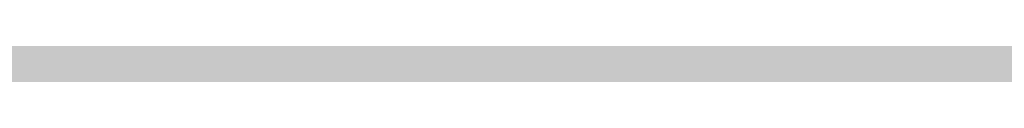
# Model space of a CAD drawing. Units: inches. Extents: x 2091 to 2899, y 967 to 2217.
# Tile 174 of 256: x 2203.151632 to 2203.161218, y 1152.24727 to 1152.24748. Entities that reach past the tile are written whole.
import ezdxf

# ---------------------------------------------------------------- set-up
doc = ezdxf.new("R2010")
doc.units = ezdxf.units.IN
doc.layers.add('A-WALL-PATT', color=141, linetype='Continuous', lineweight=13, true_color=0xadddf7)

msp = doc.modelspace()

# ---------------------------------------------------------------- hatches: boundary and pattern name
at = {"layer": 'A-WALL-PATT'}
h = msp.add_hatch(color=256, dxfattribs=at)
h.dxf.hatch_style = 1
h.paths.add_polyline_path([(2803.1436027, 2050.9190588), (2203.1436027, 2050.9190588), (2203.1436027, 1090.9190588), (2803.1436027, 1090.9190588)])
h.paths.add_polyline_path([(2635.7988501, 1147.5404649), (2674.5240524, 1147.5404649, 0.376086), (2678.5296653, 1152.8802017), (2678.5296653, 1159.5564734, 0.333335), (2674.524319, 1163.561846), (2674.524319, 1163.5618504), (2674.524319, 1192.9343904), (2635.8059707, 1192.9343904), (2597.0876225, 1192.9343904), (2597.0876225, 1163.561846, 0.333335), (2593.0822761, 1159.5564734), (2593.0822761, 1152.8802017, 0.376086), (2597.087889, 1147.5404649)], flags=0)
h.paths.add_polyline_path([(2436.0104329, 1278.2407784, 0.000483), (2435.9526433, 1278.215027, -0.001328), (2435.9356253, 1278.1116934, -0.001711), (2436.1164401, 1278.0407583, 0.002185)], flags=0)
h.paths.add_polyline_path([(2794.1436027, 1143.4190588), (2794.1436027, 1347.4190588), (2543.3701706, 1347.4190588), (2543.3701706, 1351.9190588), (2794.1436027, 1351.9190588), (2794.1436027, 1392.7135549), (2793.9473982, 1392.7135549), (2793.9473982, 1473.5368999), (2794.1436027, 1473.5368999), (2794.1436027, 1531.9190588), (2650.1436027, 1531.9190588), (2650.1436027, 1536.4190588), (2794.1436027, 1536.4190588), (2794.1436027, 1692.4190588), (2609.3756095, 1692.4190588), (2609.3756095, 1644.4190588), (2604.8756095, 1644.4190588), (2604.8756095, 1744.9190588), (2609.3756095, 1744.9190588), (2609.3756095, 1696.9190588), (2794.1436027, 1696.9190588), (2794.1436027, 1780.9190588), (2609.6436027, 1780.9190588), (2493.8756095, 1780.9190588), (2493.8756095, 1785.4190588), (2609.6436027, 1785.4190588), (2794.1436027, 1785.4190588), (2794.1436027, 1847.9388214), (2793.9512217, 1847.9388214), (2793.9512217, 1928.7621663), (2794.1436027, 1928.7621663), (2794.1436027, 1941.4190588), (2614.1436027, 1941.4190588), (2614.1436027, 1821.4190588), (2609.6436027, 1821.4190588), (2609.6436027, 1941.4190588), (2392.1436027, 1941.4190588), (2392.1436027, 1819.9190588), (2387.6436027, 1819.9190588), (2387.6436027, 1941.4190588), (2212.1436027, 1941.4190588), (2212.1436027, 1783.9190588), (2392.1436027, 1783.9190588), (2392.1436027, 1780.9190588), (2212.1436027, 1780.9190588), (2212.1436027, 1629.4190588), (2387.6436027, 1629.4190588), (2387.6436027, 1744.9190588), (2392.1436027, 1744.9190588), (2392.1436027, 1627.9190588), (2317.1436027, 1627.9190588), (2317.1436027, 1551.4190588), (2317.1436027, 1536.4190588), (2459.3835909, 1536.4190588), (2459.3835909, 1602.3964802), (2463.8835909, 1602.3964802), (2463.8835909, 1531.9190588), (2456.6436027, 1531.9190588), (2456.6436027, 1529.9190588), (2452.1436027, 1529.9190588), (2452.1436027, 1531.9190588), (2312.6436027, 1531.9190588), (2312.6436027, 1551.4190588), (2306.1436027, 1551.4190588), (2306.1436027, 1555.9190588), (2308.1436027, 1555.9190588), (2308.1436027, 1551.4190588), (2312.6436027, 1551.4190588), (2312.6436027, 1627.9190588), (2212.1436027, 1627.9190588), (2212.1436027, 1555.9190588), (2270.1436027, 1555.9190588), (2270.1436027, 1551.4190588), (2212.1436027, 1551.4190588), (2212.1436027, 1351.9190588), (2272.1436027, 1351.9190588), (2272.1436027, 1347.4190588), (2212.1436027, 1347.4190588), (2212.1436027, 1275.4190588), (2308.1436027, 1275.4190588), (2308.1436027, 1351.9190588), (2452.1436027, 1351.9190588), (2452.1436027, 1493.9190588), (2456.6436027, 1493.9190588), (2456.6436027, 1347.4190588), (2312.6436027, 1347.4190588), (2312.6436027, 1270.9190588), (2212.1436027, 1270.9190588), (2212.1436027, 1099.9190588), (2281.2375229, 1099.9190588), (2282.8710413, 1110.9138034), (2282.0083413, 1116.9966034), (2278.5577413, 1121.4204034), (2268.2056413, 1128.0562034), (2272.0876413, 1128.0562034), (2273.8129413, 1131.9270034), (2279.4203413, 1134.6919034), (2285.0278413, 1135.2449034), (2287.6158413, 1137.4568034), (2288.0471413, 1138.0098034), (2289.3411413, 1140.7747034), (2291.0665413, 1139.6687034), (2292.3605413, 1135.2449034), (2295.3798413, 1136.9038034), (2296.2425413, 1135.7979034), (2297.1052413, 1133.0330034), (2300.1246413, 1138.0098034), (2303.1439413, 1138.0098034), (2304.4379413, 1135.7979034), (2303.1439413, 1133.5860034), (2306.5946413, 1134.6919034), (2307.8887413, 1133.0330034), (2310.9080413, 1135.2449034), (2313.9274413, 1134.1389034), (2315.6268599, 1132.4271023), (2308.3200413, 1117.5496034), (2290.2038413, 1109.8079034), (2288.9098413, 1103.1721034), (2289.2723086, 1099.9190588), (2434.9182274, 1099.9190588), (2431.5932274, 1124.7880588), (2429.9302274, 1169.5530588), (2430.9271848, 1240.5196942), (2435.6589255, 1238.1861258), (2437.1352274, 1196.5540588), (2438.7982274, 1143.9730588), (2442.6782274, 1111.9980588), (2446.5582274, 1099.9190588), (2794.1436027, 1099.9190588), (2794.1436027, 1138.9190588), (2548.0324471, 1138.9190588), (2548.0324471, 1143.4190588), (2548.0324471, 1148.8190588), (2546.6684571, 1148.0315588), (2528.6856919, 1179.1786218, 0.256256), (2512.0324471, 1148.8190588), (2512.0324471, 1143.4190588), (2512.0324471, 1138.9190588), (2507.5324471, 1138.9190588), (2507.5324471, 1143.4190588), (2507.5324471, 1148.8190588, 0.256256), (2490.8792023, 1179.1786218), (2472.8964371, 1148.0315588), (2471.5324471, 1148.8190588), (2471.5324471, 1143.4190588), (2467.0324471, 1143.4190588), (2467.0324471, 1269.9457858, 0.039061), (2460.9099871, 1273.5800588), (2467.0324471, 1273.5800588), (2467.0324471, 1286.3253638, 0.014511), (2465.2161944, 1286.7619052), (2467.0324471, 1287.0525761), (2467.0324471, 1323.4190588), (2471.5324471, 1323.4190588), (2471.5324471, 1148.8190588), (2489.5324471, 1179.9959734), (2490.8964371, 1179.2084734), (2490.8792023, 1179.1786218, -0.256256), (2507.5324471, 1148.8190588), (2507.5324471, 1143.4190588), (2512.0324471, 1143.4190588), (2512.0324471, 1148.8190588, -0.256256), (2528.6856919, 1179.1786218), (2528.6684571, 1179.2084734), (2530.0324471, 1179.9959734), (2548.0324471, 1148.8190588), (2548.0324471, 1143.4190588)], flags=16)
h.paths.add_polyline_path([(2607.7685461, 1200.9450832), (2607.7685461, 1265.0306251), (2597.0876225, 1281.0520106), (2619.7845852, 1281.0520106), (2627.795278, 1337.1268598), (2635.7988501, 1337.1268598), (2643.8166634, 1337.1268598), (2651.8273562, 1281.0520106), (2674.524319, 1281.0520106), (2663.8433953, 1265.0306251), (2663.8433953, 1200.9450832), (2635.8059707, 1200.9450832)], flags=0)
edge = h.paths.add_edge_path(flags=0)
edge.add_ellipse((13303.8962153, 1272.9987247), major_axis=(-10595.3130399, 0.0000005), ratio=0.842303870086, start_angle=0.62823721906, end_angle=0.64655409989, ccw=False)
edge.add_ellipse((2711.7004495, 1156.8526781), major_axis=(2.2197691, 0), ratio=0.84230387, start_angle=111.5352435, end_angle=180.6282372, ccw=False)
edge.add_ellipse((13303.1562922, 1272.9987246), major_axis=(-10593.0263064, 0), ratio=0.842303869544, start_angle=0.52827147182, end_angle=0.64655409706, ccw=False)
edge.add_line((2710.7645961, 1175.3332951), (2710.1299858, 1175.3332951))
edge.add_ellipse((2710.1299858, 1176.5797752), major_axis=(1.4798461, 0), ratio=0.84230387, start_angle=180, end_angle=270, ccw=False)
edge.add_line((2708.6501397, 1176.5797752), (2708.6501397, 1200.7829144))
edge.add_ellipse((2710.1299858, 1200.7829144), major_axis=(1.4798461, 0), ratio=0.84230387, start_angle=90, end_angle=180, ccw=False)
edge.add_line((2710.1299858, 1202.0293944), (2710.4650752, 1202.0293944))
edge.add_ellipse((13303.1562922, 1272.9987246), major_axis=(-10593.0263064, 0), ratio=0.842303869544, start_angle=-0.09022908859, end_angle=0.38386677879, ccw=False)
edge.add_ellipse((2710.1299858, 1290.9270308), major_axis=(-1.4798461, 0), ratio=0.84230387, start_angle=0, end_angle=90, ccw=False)
edge.add_line((2708.6501397, 1290.9270308), (2708.6501397, 1315.13017))
edge.add_ellipse((2710.1299858, 1315.13017), major_axis=(-1.4798461, 0), ratio=0.84230387, start_angle=-90, end_angle=0, ccw=False)
edge.add_line((2710.1299858, 1316.3766501), (2710.7063141, 1316.3766501))
edge.add_ellipse((3238.4017202, 1296.2895655), major_axis=(528.2339998, 0), ratio=0.84230386954, start_angle=176.349572414, end_angle=177.820049686, ccw=False)
edge.add_ellipse((2775.0630432, 1071.4506962), major_axis=(313.3077613, 0), ratio=0.84230386954, start_angle=102.125965552, end_angle=103.780528989, ccw=False)
edge.add_ellipse((2775.0630432, 1078.3056979), major_axis=(-305.3028915, 0), ratio=0.84230386955, start_angle=-79.790461003, end_angle=-77.555372706, ccw=False)
edge.add_ellipse((2695.1417666, 1541.9753825), major_axis=(-250.9602162, 0), ratio=0.84230386954, start_angle=99.256566007, end_angle=102.554932644)
edge.add_line((2741.4103262, 1334.2142554), (2747.1325454, 1337.3784768))
edge.add_ellipse((2747.5386163, 1336.8574776), major_axis=(-0.739923, 0), ratio=0.84230387, start_angle=270, end_angle=307.9331305, ccw=False)
edge.add_ellipse((2747.5386163, 1336.8574776), major_axis=(-0.739923, 0), ratio=0.84230387, start_angle=232.0668695, end_angle=270, ccw=False)
edge.add_line((2747.9446872, 1337.3784768), (2753.6669064, 1334.2142554))
edge.add_ellipse((2799.935466, 1541.9753825), major_axis=(250.9602162, 0), ratio=0.84230386954, start_angle=257.445067356, end_angle=260.743433993)
edge.add_ellipse((2720.0141894, 1078.3056979), major_axis=(305.3028915, 0), ratio=0.84230386954, start_angle=77.555372707, end_angle=79.790461003, ccw=False)
edge.add_ellipse((2720.0141894, 1071.4506962), major_axis=(-313.3077613, 0), ratio=0.84230386954, start_angle=256.219471011, end_angle=257.874034448, ccw=False)
edge.add_ellipse((2256.6755124, 1296.2895655), major_axis=(-528.2339998, 0), ratio=0.84230386954, start_angle=182.179950314, end_angle=183.650427586, ccw=False)
edge.add_line((2784.3709184, 1316.3766501), (2784.9472468, 1316.3766501))
edge.add_ellipse((2784.9472468, 1315.13017), major_axis=(1.4798461, 0), ratio=0.84230387, start_angle=0, end_angle=90, ccw=False)
edge.add_line((2786.4270928, 1315.13017), (2786.4270928, 1290.9270308))
edge.add_ellipse((2784.9472468, 1290.9270308), major_axis=(1.4798461, 0), ratio=0.84230387, start_angle=270, end_angle=360, ccw=False)
edge.add_ellipse((-7808.0790596, 1272.9987246), major_axis=(10593.0263063, 0), ratio=0.842303869544, start_angle=-0.38386677879, end_angle=0.09022908859, ccw=False)
edge.add_line((2784.6121574, 1202.0293944), (2784.9472468, 1202.0293944))
edge.add_ellipse((2784.9472468, 1200.7829144), major_axis=(1.4798461, 0), ratio=0.84230387, start_angle=0, end_angle=90, ccw=False)
edge.add_line((2786.4270928, 1200.7829144), (2786.4270928, 1176.5797752))
edge.add_ellipse((2784.9472468, 1176.5797752), major_axis=(-1.4798461, 0), ratio=0.84230387, start_angle=90, end_angle=180, ccw=False)
edge.add_line((2784.9472468, 1175.3332951), (2784.3126365, 1175.3332951))
edge.add_ellipse((-7808.0790596, 1272.9987246), major_axis=(10593.0263063, 0), ratio=0.842303869544, start_angle=-0.61864319632, end_angle=-0.52827147182, ccw=False)
edge.add_ellipse((2783.3767831, 1156.8526781), major_axis=(-2.2197691, 0), ratio=0.84230387, start_angle=179.3717628, end_angle=248.4647566, ccw=False)
edge.add_ellipse((-7808.8189826, 1272.9987246), major_axis=(-10595.3130398, 0.0000036), ratio=0.842303865762, start_angle=179.3534459226, end_angle=179.37176280343, ccw=False)
edge.add_ellipse((2780.2973026, 1153.500793), major_axis=(-5.2464256, 0), ratio=0.84230387, start_angle=90, end_angle=179.3534459, ccw=False)
edge.add_line((2780.2973026, 1149.0817084), (2714.77993, 1149.0817084))
edge.add_ellipse((2714.77993, 1153.500793), major_axis=(5.2464256, 0), ratio=0.84230387, start_angle=180.6465541, end_angle=270, ccw=False)
edge = h.paths.add_edge_path(flags=0)
edge.add_line((2718.1873674, 1151.0078329), (2718.1873674, 1170.4723638))
edge.add_ellipse((2721.1470595, 1170.4723638), major_axis=(-2.9596921, 0), ratio=0.84230387, start_angle=-90, end_angle=0, ccw=False)
edge.add_line((2721.1470595, 1172.965324), (2773.9301731, 1172.965324))
edge.add_ellipse((2773.9301731, 1170.4723638), major_axis=(-2.9596921, 0), ratio=0.84230387, start_angle=180, end_angle=270, ccw=False)
edge.add_line((2776.8898652, 1170.4723638), (2776.8898652, 1151.0078329))
edge.add_line((2776.8898652, 1151.0078329), (2718.1873674, 1151.0078329))
edge = h.paths.add_edge_path(flags=0)
edge.add_line((2718.1873674, 1180.2341502), (2718.1873674, 1199.0578342))
edge.add_ellipse((2747.5386163, 1320.3986402), major_axis=(147.0179239, 0), ratio=0.84230386954, start_angle=256.40186531, end_angle=283.59813469)
edge.add_line((2776.8898652, 1199.0578342), (2776.8898652, 1180.2341502))
edge.add_ellipse((2747.5386163, 1301.5749562), major_axis=(147.0179239, 0), ratio=0.84230386954, start_angle=256.40186531, end_angle=283.59813469, ccw=False)
edge = h.paths.add_edge_path(flags=0)
edge.add_ellipse((13303.1562922, 1272.9987246), major_axis=(-10591.5464603, 0), ratio=0.842303869555, start_angle=0.05559431352, end_angle=0.37776419393, ccw=False)
edge.add_line((2711.6168595, 1262.7217103), (2715.6674076, 1249.4953957))
edge.add_ellipse((6413.8919626, 1241.691919), major_axis=(-3698.2361592, 0), ratio=0.842303869547, start_angle=-0.120897369, end_angle=0.3640763489)
edge.add_line((2715.7610383, 1218.1924547), (2711.9343065, 1203.167361))
edge = h.paths.add_edge_path(flags=0)
edge.add_line((2718.1873674, 1251.074566), (2716.0024854, 1267.4504351))
edge.add_ellipse((2742.1511746, 1202.1895399), major_axis=(81.7725845, 0), ratio=0.8423038695, start_angle=94.277420963, end_angle=111.834953797, ccw=False)
edge.add_line((2737.0097482, 1270.9306255), (2758.0674844, 1270.9306255))
edge.add_ellipse((2752.926058, 1202.1895399), major_axis=(81.7725845, 0), ratio=0.8423038695, start_angle=68.165046203, end_angle=85.722579037, ccw=False)
edge.add_line((2779.0747472, 1267.4504351), (2776.8898652, 1251.074566))
edge.add_ellipse((2750.3380588, 1187.8853558), major_axis=(79.5796641, 0), ratio=0.8423038695, start_angle=67.208085122, end_angle=85.129930403)
edge.add_line((2756.0346562, 1254.7436557), (2739.0425764, 1254.7436557))
edge.add_ellipse((2744.7391738, 1187.8853558), major_axis=(79.5796641, 0), ratio=0.8423038695, start_angle=94.870069597, end_angle=112.791914878)
edge = h.paths.add_edge_path(flags=0)
edge.add_line((2783.1429261, 1203.167361), (2779.3161943, 1218.1924547))
edge.add_ellipse((-918.81473, 1241.691919), major_axis=(3698.2361592, 0), ratio=0.842303869546, start_angle=-0.3640763489, end_angle=0.120897369)
edge.add_line((2779.409825, 1249.4953957), (2783.4603731, 1262.7217103))
edge.add_ellipse((-7808.0790596, 1272.9987246), major_axis=(-10591.5464603, 0), ratio=0.84230386954, start_angle=179.6222358061, end_angle=179.94440568651, ccw=False)
edge = h.paths.add_edge_path(flags=0)
edge.add_ellipse((2734.2008921, 1286.6904402), major_axis=(-0.3566086, 6.3400775), ratio=0.603833576, start_angle=89.00201428, end_angle=253.65740805, ccw=False)
edge.add_line((2730.3690013, 1286.5418057), (2730.3690013, 1301.3519803))
edge.add_line((2730.3690013, 1301.3519803), (2735.9133107, 1305.2148028))
edge.add_ellipse((2736.3849168, 1304.7345612), major_axis=(0.739923, 0), ratio=0.84230387, start_angle=90, end_angle=134.4802109, ccw=False)
edge.add_line((2736.3849168, 1305.3578013), (2738.0327829, 1305.3578013))
edge.add_line((2738.0327829, 1305.3578013), (2738.0327829, 1307.7079274))
edge.add_ellipse((2794.201642, 1307.7079274), major_axis=(56.168859, 0), ratio=0.8423038695, start_angle=150.5614304, end_angle=180, ccw=False)
edge.add_ellipse((2700.8755906, 1307.7079274), major_axis=(-56.168859, 0), ratio=0.8423038695, start_angle=180, end_angle=209.4385696, ccw=False)
edge.add_line((2757.0444497, 1307.7079274), (2757.0444497, 1305.3578013))
edge.add_line((2757.0444497, 1305.3578013), (2758.6923157, 1305.3578013))
edge.add_ellipse((2758.6923157, 1304.7345612), major_axis=(-0.739923, 0), ratio=0.84230387, start_angle=225.5197891, end_angle=270, ccw=False)
edge.add_line((2759.1639219, 1305.2148028), (2764.7082312, 1301.3519803))
edge.add_line((2764.7082312, 1301.3519803), (2764.7082312, 1286.5418057))
edge.add_ellipse((2760.8763405, 1286.6904402), major_axis=(0.3566086, 6.3400775), ratio=0.603833576, start_angle=106.34259195, end_angle=270.99798572, ccw=False)
edge.add_line((2757.0444497, 1285.7970896), (2757.0444497, 1307.7079274))
edge.add_ellipse((2700.8755906, 1307.7079274), major_axis=(-56.168859, 0), ratio=0.8423038695, start_angle=180, end_angle=209.4385696)
edge.add_ellipse((2794.201642, 1307.7079274), major_axis=(56.168859, 0), ratio=0.8423038695, start_angle=150.5614304, end_angle=180)
edge.add_line((2738.0327829, 1307.7079274), (2738.0327829, 1285.7970896))
h.paths.add_polyline_path([(2417.8122727, 1104.449704), (2413.4922727, 1102.529704), (2410.6122727, 1103.969704), (2409.1722727, 1106.369704), (2407.2522727, 1107.329704), (2406.2922727, 1109.729704), (2405.3322727, 1114.049704), (2405.3322727, 1117.889704), (2406.2922727, 1120.129704), (2407.2522727, 1119.809704), (2408.8483218, 1118.3276585), (2410.1739451, 1119.4241703), (2410.2112727, 1120.405704), (2411.0407305, 1121.4190541), (2410.6992727, 1119.858704), (2410.1739451, 1119.4241703), (2410.0884515, 1117.1761095), (2411.1328361, 1116.2063237), (2413.9722727, 1119.329704), (2416.8522727, 1120.769704), (2416.8697209, 1120.7987842), (2417.0350713, 1119.4051162), (2417.8962134, 1118.1433844), (2418.2922727, 1118.369704), (2419.5444467, 1120.0392692), (2419.3609153, 1118.387487), (2419.0321078, 1119.3561507), (2418.3989394, 1118.5119262), (2419.2522727, 1114.529704), (2418.7940909, 1107.1987949)], flags=0)
h.paths.add_polyline_path([(2508.8701706, 1347.4190588), (2508.3701706, 1347.4190588), (2508.3701706, 1351.9190588), (2508.8701706, 1351.9190588)], flags=0)
h.paths.add_polyline_path([(2473.3701706, 1347.4190588), (2472.3701706, 1347.4190588), (2467.8701706, 1347.4190588), (2467.8701706, 1455.4190588), (2472.3701706, 1455.4190588), (2472.3701706, 1352.4190588), (2473.3701706, 1352.4190588)], flags=0)
h.paths.add_polyline_path([(2352.106244, 1217.4461971), (2349.226244, 1218.8861971), (2347.786244, 1221.2861971), (2345.866244, 1222.2461971), (2344.906244, 1224.6461971), (2343.946244, 1228.9661971), (2343.946244, 1232.8061971), (2344.906244, 1235.0461971), (2345.866244, 1234.7261971), (2347.4622931, 1233.2441515), (2348.7879164, 1234.3406634), (2348.825244, 1235.3221971), (2349.6547018, 1236.3355471), (2349.313244, 1234.7751971), (2348.7879164, 1234.3406634), (2348.7024228, 1232.0926025), (2349.7468074, 1231.1228168), (2352.586244, 1234.2461971), (2355.466244, 1235.6861971), (2355.4836921, 1235.7152773), (2355.6490426, 1234.3216093), (2356.5101846, 1233.0598774), (2356.906244, 1233.2861971), (2358.1584179, 1234.9557623), (2357.9748866, 1233.3039801), (2357.6460791, 1234.2726438), (2357.0129107, 1233.4284193), (2357.866244, 1229.4461971), (2357.4080622, 1222.115288), (2356.426244, 1219.3661971)], flags=0)
h.paths.add_polyline_path([(2348.2967999, 1112.2244204), (2347.0137999, 1112.3104204), (2345.5297999, 1114.1274204), (2345.7317999, 1115.8584204), (2346.8117999, 1116.9824204), (2346.8117999, 1114.6464204), (2345.8667999, 1114.2144204), (2346.8797999, 1114.3004204)], flags=0)
h.paths.add_polyline_path([(2347.0137999, 1110.9264204), (2346.2717999, 1110.4934204), (2346.6097999, 1111.1864204)], flags=0)
h.paths.add_polyline_path([(2345.8667999, 1118.1944204), (2345.5297999, 1117.3294204), (2343.7077999, 1118.0214204), (2344.3827999, 1118.6264204)], flags=0)
h.paths.add_polyline_path([(2346.6767999, 1109.2824204), (2346.0697999, 1108.0714204), (2345.8667999, 1110.0614204)], flags=0)
h.paths.add_polyline_path([(2345.0567999, 1119.7514204), (2343.6397999, 1119.7514204), (2343.9777999, 1121.1354204)], flags=0)
h.paths.add_polyline_path([(2345.2597999, 1116.5504204), (2345.1247999, 1115.8584204), (2344.9217999, 1115.6854204), (2344.7197999, 1116.3774204)], flags=0)
h.paths.add_polyline_path([(2345.6647999, 1112.3104204), (2345.4617999, 1111.5324204), (2344.0447999, 1111.9644204), (2344.6517999, 1112.5704204)], flags=0)
h.paths.add_polyline_path([(2345.1917999, 1113.3494204), (2344.4497999, 1113.8684204), (2344.7197999, 1114.3874204)], flags=0)
h.paths.add_polyline_path([(2344.6517999, 1116.8094204), (2344.1797999, 1115.6854204), (2344.6517999, 1115.3394204), (2343.9097999, 1114.9064204), (2343.0327999, 1115.9444204), (2343.6397999, 1116.4634204)], flags=0)
h.paths.add_polyline_path([(2345.8667999, 1106.6864204), (2344.9897999, 1105.5624204), (2344.5167999, 1106.6004204)], flags=0)
h.paths.add_polyline_path([(2344.8547999, 1110.0614204), (2344.5167999, 1109.2824204), (2344.1127999, 1109.7154204)], flags=0)
h.paths.add_polyline_path([(2344.0447999, 1113.5224204), (2343.4377999, 1113.0894204), (2342.7627999, 1113.9544204)], flags=0)
h.paths.add_polyline_path([(2344.3147999, 1111.0124204), (2342.9647999, 1110.3204204), (2342.9647999, 1111.0994204)], flags=0)
h.paths.add_polyline_path([(2345.1247999, 1104.6974204), (2344.5847999, 1103.7454204), (2344.4497999, 1104.2644204)], flags=0)
h.paths.add_polyline_path([(2342.8297999, 1121.2224204), (2341.7497999, 1120.5304204), (2340.5357999, 1121.0494204), (2340.1307999, 1121.8284204), (2340.6707999, 1122.9524204), (2341.1427999, 1121.8284204), (2341.6147999, 1122.0014204)], flags=0)
h.paths.add_polyline_path([(2342.9647999, 1119.7514204), (2343.0327999, 1118.4534204), (2342.0877999, 1118.0214204), (2342.0197999, 1119.4914204)], flags=0)
h.paths.add_polyline_path([(2342.6947999, 1116.8964204), (2341.9527999, 1116.6364204), (2342.0197999, 1117.3294204)], flags=0)
h.paths.add_polyline_path([(2343.0327999, 1112.2244204), (2342.0197999, 1111.7914204), (2341.5477999, 1112.2244204), (2342.3577999, 1113.3494204)], flags=0)
h.paths.add_polyline_path([(2343.7747999, 1104.4374204), (2342.6277999, 1102.8804204), (2342.6947999, 1104.6104204), (2343.4377999, 1105.1294204)], flags=0)
h.paths.add_polyline_path([(2342.0197999, 1115.0794204), (2340.8057999, 1115.5124204), (2340.9407999, 1116.3774204)], flags=0)
h.paths.add_polyline_path([(2341.4807999, 1120.0974204), (2341.4807999, 1119.4054204), (2341.0757999, 1119.5784204), (2341.1427999, 1120.0974204)], flags=0)
h.paths.add_polyline_path([(2341.8177999, 1114.4734204), (2340.9407999, 1113.0894204), (2340.8057999, 1114.5604204)], flags=0)
h.paths.add_polyline_path([(2341.1427999, 1118.5404204), (2340.9407999, 1116.9824204), (2339.0507999, 1117.6754204), (2339.0507999, 1118.6264204)], flags=0)
h.paths.add_polyline_path([(2342.6947999, 1101.6684204), (2341.9527999, 1101.8414204), (2342.5597999, 1102.3614204)], flags=0)
h.paths.add_polyline_path([(2340.3327999, 1119.6654204), (2338.4437999, 1119.5784204), (2337.9037999, 1120.3574204), (2339.6577999, 1120.6164204)], flags=0)
h.paths.add_polyline_path([(2340.3327999, 1115.3394204), (2340.0627999, 1113.6954204), (2339.3877999, 1115.3394204)], flags=0)
h.paths.add_polyline_path([(2341.8177999, 1103.8314204), (2341.5477999, 1102.8804204), (2341.1427999, 1103.6584204)], flags=0)
h.paths.add_polyline_path([(2339.0507999, 1122.8664204), (2337.2957999, 1121.8284204), (2337.0937999, 1123.1254204), (2337.7687999, 1123.8184204)], flags=0)
h.paths.add_polyline_path([(2339.1177999, 1121.7414204), (2338.8477999, 1121.2224204), (2338.1737999, 1121.0494204), (2338.3757999, 1121.5684204)], flags=0)
h.paths.add_polyline_path([(2339.1857999, 1119.3194204), (2338.6457999, 1118.7134204), (2338.2407999, 1118.1074204), (2338.2407999, 1118.8864204)], flags=0)
h.paths.add_polyline_path([(2341.1427999, 1101.9284204), (2340.6027999, 1101.2364204), (2340.0627999, 1101.8414204), (2340.6027999, 1102.3614204)], flags=0)
h.paths.add_polyline_path([(2337.6337999, 1117.7614204), (2336.6207999, 1118.2804204), (2337.2957999, 1118.9724204)], flags=0)
h.paths.add_polyline_path([(2336.8237999, 1119.5784204), (2334.7987999, 1118.9724204), (2335.2037999, 1120.3574204), (2336.5537999, 1120.8764204)], flags=0)
h.paths.add_polyline_path([(2339.1177999, 1100.4574204), (2337.3637999, 1100.5434204), (2336.7557999, 1101.2364204)], flags=0)
h.paths.add_polyline_path([(2336.3507999, 1122.4334204), (2336.0137999, 1121.9144204), (2334.9337999, 1122.4334204), (2334.5287999, 1123.4714204), (2335.7437999, 1122.7794204)], flags=0)
h.paths.add_polyline_path([(2334.7317999, 1120.8764204), (2334.2587999, 1120.3574204), (2334.0567999, 1120.7894204), (2334.5967999, 1121.3084204)], flags=0)
h.paths.add_polyline_path([(2334.4617999, 1122.1744204), (2332.5717999, 1121.3084204), (2331.3567999, 1122.1744204), (2332.0997999, 1122.8664204)], flags=0)
h.paths.add_polyline_path([(2334.2587999, 1118.5404204), (2333.3817999, 1118.4534204), (2333.6517999, 1119.3194204)], flags=0)
h.paths.add_polyline_path([(2335.5417999, 1102.2744204), (2334.1917999, 1102.6204204), (2335.2717999, 1103.3124204)], flags=0)
h.paths.add_polyline_path([(2332.7067999, 1119.6654204), (2331.6947999, 1120.4434204), (2332.5047999, 1120.7894204)], flags=0)
h.paths.add_polyline_path([(2334.7317999, 1101.1494204), (2333.5167999, 1101.5824204), (2333.9887999, 1101.7554204)], flags=0)
h.paths.add_polyline_path([(2332.6397999, 1116.6364204), (2331.0867999, 1116.2904204), (2331.9647999, 1118.1944204)], flags=0)
h.paths.add_polyline_path([(2330.7497999, 1121.5684204), (2330.2767999, 1120.2704204), (2328.5227999, 1119.3194204), (2328.9947999, 1121.0494204)], flags=0)
h.paths.add_polyline_path([(2330.7497999, 1118.6264204), (2330.0077999, 1117.5024204), (2329.8727999, 1118.0214204)], flags=0)
h.paths.add_polyline_path([(2332.0997999, 1102.3614204), (2330.5467999, 1102.0144204), (2331.6947999, 1102.9664204)], flags=0)
h.paths.add_polyline_path([(2329.5347999, 1113.6084204), (2329.0627999, 1112.3104204), (2328.5897999, 1113.3494204)], flags=0)
h.paths.add_polyline_path([(2328.3877999, 1117.8484204), (2327.5097999, 1116.5504204), (2327.1727999, 1117.7614204)], flags=0)
h.paths.add_polyline_path([(2329.7377999, 1106.5134204), (2329.5347999, 1105.3024204), (2328.2527999, 1106.0814204)], flags=0)
h.paths.add_polyline_path([(2328.6577999, 1114.3874204), (2328.0497999, 1114.1274204), (2328.3197999, 1114.9064204)], flags=0)
h.paths.add_polyline_path([(2328.3197999, 1112.2244204), (2327.1057999, 1112.1374204), (2326.7007999, 1112.6564204)], flags=0)
h.paths.add_polyline_path([(2326.9027999, 1115.2524204), (2326.7007999, 1114.1274204), (2325.2157999, 1113.6084204), (2326.0927999, 1115.3394204)], flags=0)
h.paths.add_polyline_path([(2326.6327999, 1108.3304204), (2326.0927999, 1107.3794204), (2325.8907999, 1108.5034204), (2326.4977999, 1109.1094204)], flags=0)
h.paths.add_polyline_path([(2615.1436027, 1531.9190588), (2609.6436027, 1531.9190588), (2609.6436027, 1620.4190588), (2614.1436027, 1620.4190588), (2614.1436027, 1536.4190588), (2615.1436027, 1536.4190588)], flags=0)
h.paths.add_polyline_path([(2545.1436027, 1563.4190588), (2464.1436027, 1563.4190588), (2464.1436027, 1632.4190588), (2509.1436027, 1632.4190588), (2509.1436027, 1627.9190588), (2509.1436027, 1603.9190588), (2468.6436027, 1603.9190588), (2468.6436027, 1567.9190588), (2540.6436027, 1567.9190588), (2540.6436027, 1591.9190588), (2545.1436027, 1591.9190588)], flags=0)
h.paths.add_polyline_path([(2388.9690483, 1549.985735), (2357.4341811, 1549.985735), (2357.4341811, 1623.3607783), (2399.3627772, 1623.3607783), (2435.6894654, 1623.3607783), (2435.5925469, 1602.5592734), (2435.5925469, 1602.3964802), (2388.9690483, 1602.3964802)], flags=0)
h.paths.add_polyline_path([(2388.8806282, 1555.8091511), (2374.9044295, 1555.8091511), (2374.9044295, 1600.5715641), (2374.9044295, 1615.4576454), (2406.3508766, 1615.4576454), (2406.3508766, 1618.9394309), (2412.1742927, 1615.4576454), (2406.3508766, 1611.9758599), (2406.3508766, 1615.4576454), (2388.8806282, 1615.4576454)], flags=0)
h.paths.add_polyline_path([(2568.8756095, 1644.4190588), (2453.3756095, 1644.4190588), (2453.3756095, 1785.4190588), (2457.8756095, 1785.4190588), (2457.8756095, 1648.9190588), (2568.8756095, 1648.9190588)], flags=0)
h.paths.add_polyline_path([(2212.1436027, 1945.9190588), (2212.1436027, 2041.9190588), (2794.1436027, 2041.9190588), (2794.1436027, 1945.9190588)], flags=16)
h.paths.add_polyline_path([(2271.0827276, 1964.3172377), (2776.852968, 1964.3172377), (2776.852968, 2037.1696226), (2271.0827276, 2037.1696226)], flags=8)
h.paths.add_polyline_path([(2380.6492852, 1536.8241435), (2461.0408087, 1536.8241435), (2461.0408087, 1554.6525871), (2380.6492852, 1554.6525871)], flags=8)
h.paths.add_polyline_path([(2240.7557092, 1609.7254508), (2309.1858294, 1609.7254508), (2309.1858294, 1617.6982037), (2240.7557092, 1617.6982037)], flags=8)
h.paths.add_polyline_path([(2212.6772554, 1313.5041021), (2282.5915203, 1313.5041021), (2282.5915203, 1322.7452389), (2212.6772554, 1322.7452389)], flags=8)
h.paths.add_polyline_path([(2457.111976, 1114.778574), (2558.4815807, 1114.778574), (2558.4815807, 1142.2196823), (2457.111976, 1142.2196823)], flags=8)
h.paths.add_polyline_path([(2473.4423372, 1273.0100672), (2604.6412257, 1273.0100672), (2604.6412257, 1318.3469349), (2473.4423372, 1318.3469349)], flags=8)
h.paths.add_polyline_path([(2638.8763024, 1626.9774316), (2684.2503675, 1627.9767377), (2684.0384825, 1637.5974944), (2638.6644174, 1636.5981884)], flags=8)
h.paths.add_polyline_path([(2537.5905538, 1453.7934466), (2628.3895472, 1453.7934466), (2628.3895472, 1475.3448114), (2537.5905538, 1475.3448114)], flags=8)
h.paths.add_polyline_path([(2504.1376376, 1714.6323972), (2554.6471875, 1714.6323972), (2554.6471875, 1730.2377115), (2504.1376376, 1730.2377115)], flags=8)
h.paths.add_polyline_path([(2487.5011806, 1575.6518716), (2535.0971214, 1575.6518716), (2535.0971214, 1598.3776456), (2487.5011806, 1598.3776456)], flags=8)
h.paths.add_polyline_path([(2709.0994004, 1735.7102784), (2740.0166009, 1735.7102784), (2740.0166009, 1749.9376406), (2709.0994004, 1749.9376406)], flags=8)
h.paths.add_polyline_path([(2442.4384239, 1792.1716575), (2564.7288353, 1792.1716575), (2564.7288353, 1842.0001626), (2442.4384239, 1842.0001626)], flags=8)
h.paths.add_polyline_path([(2655.8158012, 1809.6440763), (2789.5201425, 1806.6937963), (2790.0849768, 1832.2916379), (2656.3806355, 1835.2419179)], flags=8)
h.paths.add_polyline_path([(2234.8426972, 1797.7201432), (2368.5928512, 1794.7688523), (2369.1607182, 1820.504132), (2235.4105642, 1823.4554229)], flags=8)
h.paths.add_polyline_path([(2245.1384659, 1644.0063348), (2398.4277329, 1640.6238997), (2398.9948417, 1666.3248199), (2245.7055747, 1669.7072549)], flags=8)
h.paths.add_polyline_path([(2306.1428474, 1431.1685186), (2413.7683138, 1428.7936873), (2414.3331481, 1454.3915289), (2306.7076817, 1456.7663602)], flags=8)
h.paths.add_polyline_path([(2306.834582, 1458.2331447), (2393.3804836, 1456.3234487), (2393.9328082, 1481.3543583), (2307.3869066, 1483.2640542)], flags=8)

doc.saveas('drawing.dxf')
